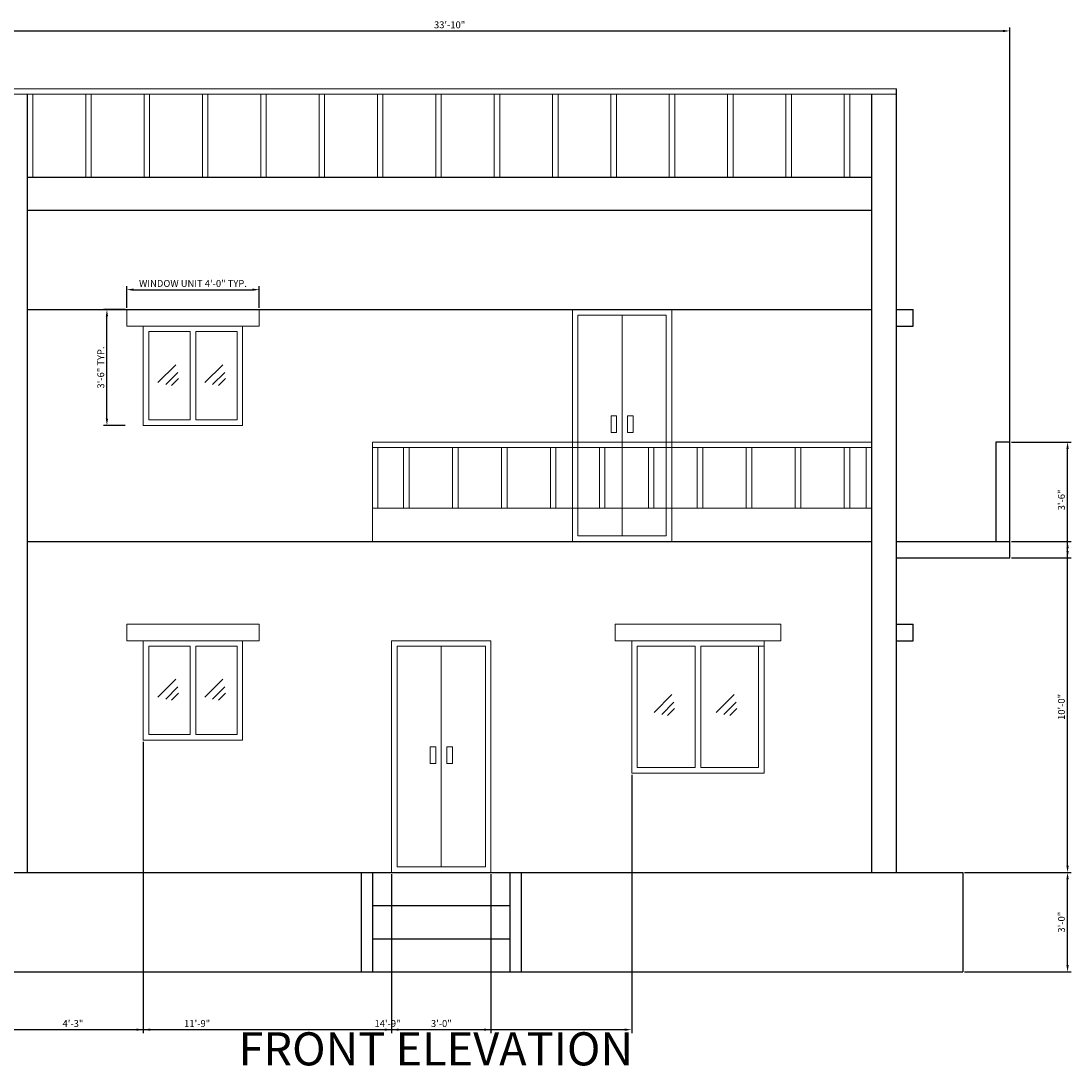
# Model space of a CAD drawing. Units: inches. Extents: x 2443635 to 2446153, y 1826255 to 1827341.
# Tile 16 of 16: x 2445772 to 2446153, y 1826829 to 1827207. Entities that reach past the tile are written whole.
import ezdxf

# ---------------------------------------------------------------- set-up
doc = ezdxf.new("R2010")
doc.units = ezdxf.units.IN
for name, color, linetype, lineweight in [('A-DIMS', 1, 'Continuous', 18), ('A-ELEV', 7, 'Continuous', 25), ('A-ELEV-DOOR', 2, 'Continuous', 18), ('A-ELEV-GLAZ', 4, 'Continuous', 18), ('A-ELEV-RAIL', 9, 'Continuous', 18), ('A-TEXT', 4, 'Continuous', 25)]:
    doc.layers.add(name, color=color, linetype=linetype, lineweight=lineweight)
doc.styles.get("Standard").update_dxf_attribs({"font": 'arial.ttf'})
doc.dimstyles.new('ISO-25', dxfattribs={"dimtxt": 2.5, "dimasz": 2.5, "dimexe": 1.25, "dimexo": 0.625, "dimtad": 1, "dimlunit": 4, "dimtxsty": 'Standard', "dimcen": 2.5, "dimadec": 0, "dimazin": 0, "dimtfac": 1, "dimtmove": 0, "dimatfit": 3, "dimfxl": 1, "dimarcsym": 0})

# ---------------------------------------------------------------- blocks, each defined once
blk = doc.blocks.new('WINDOW-36-ELEV')
at = {"transparency": 33554687}
for p, q in [((48, 42), (0, 42)), ((0, 36), (0, 42)), ((48, 36), (48, 42)), ((48, 36), (0, 36)), ((6, 0), (6, 36)), ((42, 36), (42, 0)), ((8, 2), (8, 34)), ((23, 34), (8, 34)), ((23, 2), (23, 34)), ((40, 34), (25, 34)), ((25, 2), (25, 34)), ((40, 34), (40, 2)), ((17.76, 22), (11.31, 15.54)), ((18.51, 19.22), (14.11, 14.82)), ((34.78, 22), (28.32, 15.54)), ((35.53, 19.22), (31.13, 14.82)), ((18.76, 16.98), (16.23, 14.45)), ((35.77, 16.98), (33.24, 14.45)), ((42, 0), (6, 0)), ((23, 2), (8, 2)), ((40, 2), (25, 2))]:
    blk.add_line(p, q, dxfattribs=at)
blk = doc.blocks.new('*D78')
at = {"layer": 'A-DIMS', "color": 0, "lineweight": -2, "transparency": 16777216}
for p, q in [((2445810.56, 1827103.33), (2445810.56, 1827111.15)), ((2445813.06, 1827109.9), (2445856.06, 1827109.9)), ((2445858.56, 1827103.33), (2445858.56, 1827111.15))]:
    blk.add_line(p, q, dxfattribs=at)
at = {"layer": 'A-DIMS', "color": 0, "transparency": 16777216}
for points in [[(2445813.06, 1827110.32), (2445813.06, 1827109.48), (2445810.56, 1827109.9)], [(2445856.06, 1827110.32), (2445856.06, 1827109.48), (2445858.56, 1827109.9)]]:
    blk.add_solid(points, dxfattribs=at)
at = {"layer": 'Defpoints', "color": 0, "transparency": 16777216}
for p in [(2445858.56, 1827109.9), (2445810.56, 1827102.7), (2445858.56, 1827102.7)]:
    blk.add_point(p, dxfattribs=at)
at = {"layer": 'A-DIMS', "color": 0, "transparency": 16777216, "insert": (2445834.56, 1827111.82), "char_height": 2.5, "attachment_point": 5}
blk.add_mtext('WINDOW UNIT 4\'-0" TYP.', dxfattribs=at)
blk = doc.blocks.new('*D79')
at = {"layer": 'A-DIMS', "color": 0, "lineweight": -2, "transparency": 16777216}
for p, q in [((2445809.93, 1827102.7), (2445802.11, 1827102.7)), ((2445803.36, 1827063.2), (2445803.36, 1827100.2)), ((2445809.93, 1827060.7), (2445802.11, 1827060.7))]:
    blk.add_line(p, q, dxfattribs=at)
at = {"layer": 'A-DIMS', "color": 0, "transparency": 16777216}
for points in [[(2445802.94, 1827100.2), (2445803.78, 1827100.2), (2445803.36, 1827102.7)], [(2445802.94, 1827063.2), (2445803.78, 1827063.2), (2445803.36, 1827060.7)]]:
    blk.add_solid(points, dxfattribs=at)
at = {"layer": 'Defpoints', "color": 0, "transparency": 16777216}
for p in [(2445803.36, 1827102.7), (2445810.56, 1827102.7), (2445810.56, 1827060.7)]:
    blk.add_point(p, dxfattribs=at)
at = {"layer": 'A-DIMS', "color": 0, "transparency": 16777216, "insert": (2445801.46, 1827081.7), "char_height": 2.5, "attachment_point": 5, "rotation": 90}
blk.add_mtext('3\'-6" TYP.', dxfattribs=at)
blk = doc.blocks.new('*D107')
at = {"layer": 'A-DIMS', "color": 0, "lineweight": -2, "transparency": 16777216}
for p, q in [((2445724.56, 1827013.33), (2445724.56, 1827204.9)), ((2446130.56, 1827013.33), (2446130.56, 1827204.9)), ((2445727.06, 1827203.65), (2446128.06, 1827203.65))]:
    blk.add_line(p, q, dxfattribs=at)
at = {"layer": 'A-DIMS', "color": 0, "transparency": 16777216}
for points in [[(2445727.06, 1827204.07), (2445727.06, 1827203.23), (2445724.56, 1827203.65)], [(2446128.06, 1827204.07), (2446128.06, 1827203.23), (2446130.56, 1827203.65)]]:
    blk.add_solid(points, dxfattribs=at)
at = {"layer": 'Defpoints', "color": 0, "transparency": 16777216}
for p in [(2446130.56, 1827203.65), (2445724.56, 1827012.7), (2446130.56, 1827012.7)]:
    blk.add_point(p, dxfattribs=at)
at = {"layer": 'A-DIMS', "color": 0, "transparency": 16777216, "insert": (2445927.56, 1827205.55), "char_height": 2.5, "attachment_point": 5}
blk.add_mtext('33\'-10"', dxfattribs=at)
blk = doc.blocks.new('*D109')
at = {"layer": 'A-DIMS', "color": 0, "lineweight": -2, "transparency": 16777216}
for p, q in [((2445765.56, 1826898.08), (2445765.56, 1826840.5)), ((2445906.56, 1826898.08), (2445906.56, 1826840.5)), ((2445768.06, 1826841.75), (2445904.06, 1826841.75))]:
    blk.add_line(p, q, dxfattribs=at)
at = {"layer": 'A-DIMS', "color": 0, "transparency": 16777216}
for points in [[(2445768.06, 1826842.17), (2445768.06, 1826841.33), (2445765.56, 1826841.75)], [(2445904.06, 1826842.17), (2445904.06, 1826841.33), (2445906.56, 1826841.75)]]:
    blk.add_solid(points, dxfattribs=at)
at = {"layer": 'Defpoints', "color": 0, "transparency": 16777216}
for p in [(2445765.56, 1826898.7), (2445906.56, 1826898.7), (2445906.56, 1826841.75)]:
    blk.add_point(p, dxfattribs=at)
at = {"layer": 'A-DIMS', "color": 0, "transparency": 16777216, "insert": (2445836.06, 1826843.65), "char_height": 2.5, "attachment_point": 5}
blk.add_mtext('11\'-9"', dxfattribs=at)
blk = doc.blocks.new('*D110')
at = {"layer": 'A-DIMS', "color": 0, "lineweight": -2, "transparency": 16777216}
for p, q in [((2445906.56, 1826898.08), (2445906.56, 1826840.5)), ((2445942.56, 1826898.08), (2445942.56, 1826840.5)), ((2445909.06, 1826841.75), (2445940.06, 1826841.75))]:
    blk.add_line(p, q, dxfattribs=at)
at = {"layer": 'A-DIMS', "color": 0, "transparency": 16777216}
for points in [[(2445909.06, 1826842.17), (2445909.06, 1826841.33), (2445906.56, 1826841.75)], [(2445940.06, 1826842.17), (2445940.06, 1826841.33), (2445942.56, 1826841.75)]]:
    blk.add_solid(points, dxfattribs=at)
at = {"layer": 'Defpoints', "color": 0, "transparency": 16777216}
for p in [(2445906.56, 1826898.7), (2445942.56, 1826898.7), (2445942.56, 1826841.75)]:
    blk.add_point(p, dxfattribs=at)
at = {"layer": 'A-DIMS', "color": 0, "transparency": 16777216, "insert": (2445924.56, 1826843.65), "char_height": 2.5, "attachment_point": 5}
blk.add_mtext('3\'-0"', dxfattribs=at)
blk = doc.blocks.new('*D111')
at = {"layer": 'A-DIMS', "color": 0, "lineweight": -2, "transparency": 16777216}
for p, q in [((2445816.56, 1826946.08), (2445816.56, 1826840.5)), ((2445765.56, 1826898.08), (2445765.56, 1826840.5)), ((2445768.06, 1826841.75), (2445814.06, 1826841.75))]:
    blk.add_line(p, q, dxfattribs=at)
at = {"layer": 'A-DIMS', "color": 0, "transparency": 16777216}
for points in [[(2445768.06, 1826842.17), (2445768.06, 1826841.33), (2445765.56, 1826841.75)], [(2445814.06, 1826842.17), (2445814.06, 1826841.33), (2445816.56, 1826841.75)]]:
    blk.add_solid(points, dxfattribs=at)
at = {"layer": 'Defpoints', "color": 0, "transparency": 16777216}
for p in [(2445816.56, 1826946.7), (2445765.56, 1826898.7), (2445816.56, 1826841.75)]:
    blk.add_point(p, dxfattribs=at)
at = {"layer": 'A-DIMS', "color": 0, "transparency": 16777216, "insert": (2445791.06, 1826843.65), "char_height": 2.5, "attachment_point": 5}
blk.add_mtext('4\'-3"', dxfattribs=at)
blk = doc.blocks.new('*D112')
at = {"layer": 'A-DIMS', "color": 0, "lineweight": -2, "transparency": 16777216}
for p, q in [((2445816.56, 1826946.08), (2445816.56, 1826840.5)), ((2445993.56, 1826934.08), (2445993.56, 1826840.5)), ((2445819.06, 1826841.75), (2445991.06, 1826841.75))]:
    blk.add_line(p, q, dxfattribs=at)
at = {"layer": 'A-DIMS', "color": 0, "transparency": 16777216}
for points in [[(2445819.06, 1826842.17), (2445819.06, 1826841.33), (2445816.56, 1826841.75)], [(2445991.06, 1826842.17), (2445991.06, 1826841.33), (2445993.56, 1826841.75)]]:
    blk.add_solid(points, dxfattribs=at)
at = {"layer": 'Defpoints', "color": 0, "transparency": 16777216}
for p in [(2445816.56, 1826946.7), (2445993.56, 1826934.7), (2445993.56, 1826841.75)]:
    blk.add_point(p, dxfattribs=at)
at = {"layer": 'A-DIMS', "color": 0, "transparency": 16777216, "insert": (2445905.06, 1826843.65), "char_height": 2.5, "attachment_point": 5}
blk.add_mtext('14\'-9"', dxfattribs=at)
blk = doc.blocks.new('*D113')
at = {"layer": 'A-DIMS', "color": 0, "lineweight": -2, "transparency": 16777216}
for p, q in [((2446114.18, 1826898.7), (2446152.76, 1826898.7)), ((2446151.51, 1826865.2), (2446151.51, 1826896.2)), ((2446114.18, 1826862.7), (2446152.76, 1826862.7))]:
    blk.add_line(p, q, dxfattribs=at)
at = {"layer": 'A-DIMS', "color": 0, "transparency": 16777216}
for points in [[(2446151.09, 1826896.2), (2446151.93, 1826896.2), (2446151.51, 1826898.7)], [(2446151.09, 1826865.2), (2446151.93, 1826865.2), (2446151.51, 1826862.7)]]:
    blk.add_solid(points, dxfattribs=at)
at = {"layer": 'Defpoints', "color": 0, "transparency": 16777216}
for p in [(2446113.56, 1826898.7), (2446151.51, 1826898.7), (2446113.56, 1826862.7)]:
    blk.add_point(p, dxfattribs=at)
at = {"layer": 'A-DIMS', "color": 0, "transparency": 16777216, "insert": (2446149.61, 1826880.7), "char_height": 2.5, "attachment_point": 5, "rotation": 90}
blk.add_mtext('3\'-0"', dxfattribs=at)
blk = doc.blocks.new('*D114')
at = {"layer": 'A-DIMS', "color": 0, "lineweight": -2, "transparency": 16777216}
for p, q in [((2446131.18, 1827054.7), (2446152.76, 1827054.7)), ((2446151.51, 1827015.2), (2446151.51, 1827052.2)), ((2446131.18, 1827012.7), (2446152.76, 1827012.7))]:
    blk.add_line(p, q, dxfattribs=at)
at = {"layer": 'A-DIMS', "color": 0, "transparency": 16777216}
for points in [[(2446151.09, 1827052.2), (2446151.93, 1827052.2), (2446151.51, 1827054.7)], [(2446151.09, 1827015.2), (2446151.93, 1827015.2), (2446151.51, 1827012.7)]]:
    blk.add_solid(points, dxfattribs=at)
at = {"layer": 'Defpoints', "color": 0, "transparency": 16777216}
for p in [(2446130.56, 1827054.7), (2446151.51, 1827054.7), (2446130.56, 1827012.7)]:
    blk.add_point(p, dxfattribs=at)
at = {"layer": 'A-DIMS', "color": 0, "transparency": 16777216, "insert": (2446149.61, 1827033.7), "char_height": 2.5, "attachment_point": 5, "rotation": 90}
blk.add_mtext('3\'-6"', dxfattribs=at)
blk = doc.blocks.new('*D115')
at = {"layer": 'A-DIMS', "color": 0, "lineweight": -2, "transparency": 16777216}
for p, q in [((2446131.18, 1827018.7), (2446152.76, 1827018.7)), ((2446151.51, 1826901.2), (2446151.51, 1827016.2)), ((2446114.18, 1826898.7), (2446152.76, 1826898.7))]:
    blk.add_line(p, q, dxfattribs=at)
at = {"layer": 'A-DIMS', "color": 0, "transparency": 16777216}
for points in [[(2446151.09, 1827016.2), (2446151.93, 1827016.2), (2446151.51, 1827018.7)], [(2446151.09, 1826901.2), (2446151.93, 1826901.2), (2446151.51, 1826898.7)]]:
    blk.add_solid(points, dxfattribs=at)
at = {"layer": 'Defpoints', "color": 0, "transparency": 16777216}
for p in [(2446130.56, 1827018.7), (2446151.51, 1827018.7), (2446113.56, 1826898.7)]:
    blk.add_point(p, dxfattribs=at)
at = {"layer": 'A-DIMS', "color": 0, "transparency": 16777216, "insert": (2446149.61, 1826958.7), "char_height": 2.5, "attachment_point": 5, "rotation": 90}
blk.add_mtext('10\'-0"', dxfattribs=at)

msp = doc.modelspace()

# ---------------------------------------------------------------- linework, layer by layer
at = {"layer": 'A-ELEV'}
for p, q in [((2446089.56, 1826898.701), (2446089.56, 1827182.701)), ((2445774.56, 1826898.701), (2445774.56, 1827180.701)), ((2446080.56, 1826898.701), (2446080.56, 1827180.701)), ((2445858.56, 1827102.701), (2446080.56, 1827102.701)), ((2445741.56, 1826898.701), (2446113.56, 1826898.701)), ((2445895.56, 1826898.701), (2445895.56, 1826862.701)), ((2445899.56, 1826898.701), (2445899.56, 1826862.701)), ((2445949.56, 1826862.701), (2445949.56, 1826898.701)), ((2445953.56, 1826862.701), (2445953.56, 1826898.701)), ((2445899.56, 1826886.701), (2445949.56, 1826886.701)), ((2445899.56, 1826874.701), (2445949.56, 1826874.701)), ((2445741.56, 1826862.701), (2446113.56, 1826862.701))]:
    msp.add_line(p, q, dxfattribs=at)
at = {"layer": 'A-ELEV', "transparency": 33554687}
for p, q in [((2445774.56, 1827150.701), (2446080.56, 1827150.701)), ((2445774.56, 1827138.701), (2446080.56, 1827138.701)), ((2445774.56, 1827102.701), (2445810.56, 1827102.701)), ((2445774.56, 1827102.701), (2446080.56, 1827102.701)), ((2446089.56, 1827102.701), (2446095.56, 1827102.701)), ((2446095.56, 1827096.701), (2446095.56, 1827102.701)), ((2446089.56, 1827096.701), (2446095.56, 1827096.701)), ((2446130.56, 1827054.701), (2446125.56, 1827054.701)), ((2446125.56, 1827054.701), (2446125.56, 1827018.701)), ((2446130.56, 1827012.701), (2446130.56, 1827054.701)), ((2445774.56, 1827018.701), (2446080.56, 1827018.701)), ((2446089.56, 1827018.701), (2446130.56, 1827018.701)), ((2446089.56, 1827012.701), (2446130.56, 1827012.701)), ((2446089.56, 1826988.701), (2446095.56, 1826988.701)), ((2446095.56, 1826982.701), (2446095.56, 1826988.701)), ((2446089.56, 1826982.701), (2446095.56, 1826982.701)), ((2446113.56, 1826898.701), (2446113.56, 1826862.701))]:
    msp.add_line(p, q, dxfattribs=at)
at = {"layer": 'A-ELEV-DOOR'}
for p, q in [((2445972.06, 1827054.701), (2445972.06, 1827102.701)), ((2446008.06, 1827102.701), (2445972.06, 1827102.701)), ((2446008.06, 1827054.701), (2446008.06, 1827102.701)), ((2445974.06, 1827100.701), (2446006.06, 1827100.701)), ((2445974.06, 1827054.701), (2445974.06, 1827100.701)), ((2445990.06, 1827100.701), (2445990.06, 1827054.701)), ((2446006.06, 1827054.701), (2446006.06, 1827100.701)), ((2445986.06, 1827064.201), (2445986.06, 1827058.201)), ((2445988.06, 1827064.201), (2445986.06, 1827064.201)), ((2445988.06, 1827064.201), (2445988.06, 1827058.201)), ((2445992.06, 1827064.201), (2445992.06, 1827058.201)), ((2445992.06, 1827064.201), (2445994.06, 1827064.201)), ((2445994.06, 1827064.201), (2445994.06, 1827058.201)), ((2445988.06, 1827058.201), (2445986.06, 1827058.201)), ((2445992.06, 1827058.201), (2445994.06, 1827058.201)), ((2446008.06, 1827054.701), (2445972.06, 1827054.701)), ((2445906.56, 1826898.701), (2445906.56, 1826982.701)), ((2445942.56, 1826982.701), (2445906.56, 1826982.701)), ((2445908.56, 1826900.701), (2445908.56, 1826980.701)), ((2445908.56, 1826980.701), (2445940.56, 1826980.701)), ((2445924.56, 1826980.701), (2445924.56, 1826900.701)), ((2445940.56, 1826900.701), (2445940.56, 1826980.701)), ((2445942.56, 1826898.701), (2445942.56, 1826982.701)), ((2445920.56, 1826944.201), (2445920.56, 1826938.201)), ((2445922.56, 1826944.201), (2445920.56, 1826944.201)), ((2445922.56, 1826944.201), (2445922.56, 1826938.201)), ((2445926.56, 1826944.201), (2445926.56, 1826938.201)), ((2445926.56, 1826944.201), (2445928.56, 1826944.201)), ((2445928.56, 1826944.201), (2445928.56, 1826938.201)), ((2445922.56, 1826938.201), (2445920.56, 1826938.201)), ((2445926.56, 1826938.201), (2445928.56, 1826938.201)), ((2445908.56, 1826900.701), (2445940.56, 1826900.701))]:
    msp.add_line(p, q, dxfattribs=at)
at = {"layer": 'A-ELEV-DOOR', "transparency": 33554559}
for p, q in [((2445972.06, 1827018.701), (2445972.06, 1827054.701)), ((2445974.06, 1827020.701), (2445974.06, 1827054.701)), ((2445990.06, 1827054.701), (2445990.06, 1827020.701)), ((2446006.06, 1827020.701), (2446006.06, 1827054.701)), ((2446008.06, 1827018.701), (2446008.06, 1827054.701)), ((2445972.06, 1827018.701), (2446008.06, 1827018.701)), ((2445974.06, 1827020.701), (2446006.06, 1827020.701))]:
    msp.add_line(p, q, dxfattribs=at)
at = {"layer": 'A-ELEV-GLAZ'}
for p, q in [((2445987.56, 1826988.701), (2446047.56, 1826988.701)), ((2445987.56, 1826988.701), (2445987.56, 1826982.701)), ((2446047.56, 1826982.701), (2446047.56, 1826988.701)), ((2445987.56, 1826982.701), (2446047.56, 1826982.701)), ((2445993.56, 1826934.701), (2445993.56, 1826982.701)), ((2445995.56, 1826936.701), (2445995.56, 1826980.701)), ((2445995.56, 1826980.701), (2446016.56, 1826980.701)), ((2446016.56, 1826980.701), (2446016.56, 1826936.701)), ((2446018.56, 1826980.701), (2446018.56, 1826936.701)), ((2446018.56, 1826980.701), (2446041.56, 1826980.701)), ((2446039.56, 1826936.701), (2446039.56, 1826980.701)), ((2446041.56, 1826934.701), (2446041.56, 1826982.701)), ((2446008.102, 1826963.153), (2446001.645, 1826956.696)), ((2446030.649, 1826963.153), (2446024.192, 1826956.696)), ((2446008.847, 1826960.372), (2446004.451, 1826955.977)), ((2446009.095, 1826958.138), (2446006.562, 1826955.605)), ((2446031.394, 1826960.372), (2446026.999, 1826955.977)), ((2446031.642, 1826958.138), (2446029.109, 1826955.605)), ((2445993.56, 1826934.701), (2446041.56, 1826934.701)), ((2445995.56, 1826936.701), (2446016.56, 1826936.701)), ((2446018.56, 1826936.701), (2446039.56, 1826936.701))]:
    msp.add_line(p, q, dxfattribs=at)
at = {"layer": 'A-ELEV-RAIL', "transparency": 33554687}
for p, q in [((2445765.56, 1827182.701), (2446089.56, 1827182.701)), ((2445765.56, 1827180.701), (2446089.56, 1827180.701)), ((2445774.56, 1827150.701), (2445774.56, 1827180.701)), ((2445776.56, 1827150.701), (2445776.56, 1827180.701)), ((2445795.703, 1827150.701), (2445795.703, 1827180.701)), ((2445797.703, 1827150.701), (2445797.703, 1827180.701)), ((2445816.845, 1827150.701), (2445816.845, 1827180.701)), ((2445818.845, 1827150.701), (2445818.845, 1827180.701)), ((2445837.988, 1827150.701), (2445837.988, 1827180.701)), ((2445839.988, 1827150.701), (2445839.988, 1827180.701)), ((2445859.131, 1827150.701), (2445859.131, 1827180.701)), ((2445861.131, 1827150.701), (2445861.131, 1827180.701)), ((2445880.274, 1827150.701), (2445880.274, 1827180.701)), ((2445882.274, 1827150.701), (2445882.274, 1827180.701)), ((2445901.417, 1827150.701), (2445901.417, 1827180.701)), ((2445903.417, 1827150.701), (2445903.417, 1827180.701)), ((2445922.56, 1827150.701), (2445922.56, 1827180.701)), ((2445924.56, 1827150.701), (2445924.56, 1827180.701)), ((2445943.703, 1827150.701), (2445943.703, 1827180.701)), ((2445945.703, 1827150.701), (2445945.703, 1827180.701)), ((2445964.845, 1827150.701), (2445964.845, 1827180.701)), ((2445966.845, 1827150.701), (2445966.845, 1827180.701)), ((2445985.988, 1827150.701), (2445985.988, 1827180.701)), ((2445987.988, 1827150.701), (2445987.988, 1827180.701)), ((2446007.131, 1827150.701), (2446007.131, 1827180.701)), ((2446009.131, 1827150.701), (2446009.131, 1827180.701)), ((2446028.274, 1827150.701), (2446028.274, 1827180.701)), ((2446030.274, 1827150.701), (2446030.274, 1827180.701)), ((2446049.417, 1827150.701), (2446049.417, 1827180.701)), ((2446051.417, 1827150.701), (2446051.417, 1827180.701)), ((2446070.56, 1827150.701), (2446070.56, 1827180.701)), ((2446072.56, 1827150.701), (2446072.56, 1827180.701))]:
    msp.add_line(p, q, dxfattribs=at)
at = {"layer": 'A-ELEV-RAIL'}
for p, q in [((2445899.56, 1827018.701), (2445899.56, 1827054.701)), ((2445899.56, 1827054.701), (2446080.56, 1827054.701)), ((2445899.56, 1827052.701), (2446080.56, 1827052.701)), ((2445901.56, 1827030.701), (2445901.56, 1827052.701)), ((2445910.89, 1827030.701), (2445910.89, 1827052.701)), ((2445912.89, 1827030.701), (2445912.89, 1827052.701)), ((2445928.631, 1827030.701), (2445928.631, 1827052.701)), ((2445930.631, 1827030.701), (2445930.631, 1827052.701)), ((2445946.372, 1827030.701), (2445946.372, 1827052.701)), ((2445948.372, 1827030.701), (2445948.372, 1827052.701)), ((2445964.113, 1827030.701), (2445964.113, 1827052.701)), ((2445966.113, 1827030.701), (2445966.113, 1827052.701)), ((2445981.854, 1827030.701), (2445981.854, 1827052.701)), ((2445983.854, 1827030.701), (2445983.854, 1827052.701)), ((2445999.595, 1827030.701), (2445999.595, 1827052.701)), ((2446001.595, 1827030.701), (2446001.595, 1827052.701)), ((2446017.336, 1827030.701), (2446017.336, 1827052.701)), ((2446019.336, 1827030.701), (2446019.336, 1827052.701)), ((2446035.077, 1827030.701), (2446035.077, 1827052.701)), ((2446037.077, 1827030.701), (2446037.077, 1827052.701)), ((2446052.819, 1827030.701), (2446052.819, 1827052.701)), ((2446054.819, 1827030.701), (2446054.819, 1827052.701)), ((2446070.56, 1827030.701), (2446070.56, 1827052.701)), ((2446072.56, 1827030.701), (2446072.56, 1827052.701)), ((2446078.56, 1827030.701), (2446078.56, 1827052.701)), ((2446080.56, 1827018.701), (2446080.56, 1827054.701)), ((2445899.56, 1827030.701), (2446080.56, 1827030.701))]:
    msp.add_line(p, q, dxfattribs=at)

# ---------------------------------------------------------------- block references
at = {"layer": 'A-ELEV-GLAZ', "transparency": 33554687}
for p in [(2445810.56, 1827060.701), (2445810.56, 1826946.701)]:
    msp.add_blockref('WINDOW-36-ELEV', p, dxfattribs=at)

# ---------------------------------------------------------------- texts
at = {"layer": 'A-TEXT', "transparency": 33554687, "insert": (2445851.045, 1826840.797), "char_height": 12, "attachment_point": 1}
msp.add_mtext_dynamic_manual_height_columns('FRONT ELEVATION', width=201.69861, gutter_width=12.5, heights=[0], dxfattribs=at)

# ---------------------------------------------------------------- dimensions: what is measured, and where the dimension line sits
at = {"layer": 'A-DIMS', "transparency": 33554687}
for base, p1, p2, picture, middle in [((2446130.56, 1827203.651), (2445724.56, 1827012.701), (2446130.56, 1827012.701), '*D107', (2445927.56, 1827205.553)), ((2445816.56, 1826841.751), (2445765.56, 1826898.701), (2445816.56, 1826946.701), '*D111', (2445791.06, 1826843.653)), ((2445993.56, 1826841.751), (2445816.56, 1826946.701), (2445993.56, 1826934.701), '*D112', (2445905.06, 1826843.653)), ((2445906.56, 1826841.751), (2445765.56, 1826898.701), (2445906.56, 1826898.701), '*D109', (2445836.06, 1826843.653)), ((2445942.56, 1826841.751), (2445906.56, 1826898.701), (2445942.56, 1826898.701), '*D110', (2445924.56, 1826843.653))]:
    dim = msp.add_linear_dim(base=base, p1=p1, p2=p2, dimstyle='ISO-25', override={"dimdec": 1, "dimlfac": 1, "dimrnd": 0, "dimzin": 1, "dimdsep": 46, "dimlunit": 4, "dimfrac": 2}, dxfattribs=at)
    dim.commit()
    dim.dimension.update_dxf_attribs({"geometry": picture, "text_midpoint": middle})
dim = msp.add_linear_dim(base=(2445858.56, 1827109.901), p1=(2445810.56, 1827102.701), p2=(2445858.56, 1827102.701), text='WINDOW UNIT <> TYP.', dimstyle='ISO-25', override={"dimdec": 1, "dimlfac": 1, "dimrnd": 0, "dimzin": 1, "dimdsep": 46, "dimlunit": 4, "dimfrac": 2}, dxfattribs=at)
dim.commit()
dim.dimension.update_dxf_attribs({"geometry": '*D78', "text_midpoint": (2445834.56, 1827111.82)})
dim = msp.add_linear_dim(base=(2445803.36, 1827102.701), p1=(2445810.56, 1827060.701), p2=(2445810.56, 1827102.701), angle=90, text='<> TYP.', dimstyle='ISO-25', override={"dimdec": 1, "dimlfac": 1, "dimrnd": 0, "dimzin": 1, "dimdsep": 46, "dimlunit": 4, "dimfrac": 2}, dxfattribs=at)
dim.commit()
dim.dimension.update_dxf_attribs({"geometry": '*D79', "text_midpoint": (2445801.457, 1827081.701)})
for base, p1, p2, picture, middle in [((2446151.51, 1827054.701), (2446130.56, 1827012.701), (2446130.56, 1827054.701), '*D114', (2446149.607, 1827033.701)), ((2446151.51, 1827018.701), (2446113.56, 1826898.701), (2446130.56, 1827018.701), '*D115', (2446149.608, 1826958.701)), ((2446151.51, 1826898.701), (2446113.56, 1826862.701), (2446113.56, 1826898.701), '*D113', (2446149.607, 1826880.701))]:
    dim = msp.add_linear_dim(base=base, p1=p1, p2=p2, angle=90, dimstyle='ISO-25', override={"dimdec": 1, "dimlfac": 1, "dimrnd": 0, "dimzin": 1, "dimdsep": 46, "dimlunit": 4, "dimfrac": 2}, dxfattribs=at)
    dim.commit()
    dim.dimension.update_dxf_attribs({"geometry": picture, "text_midpoint": middle})

doc.saveas('drawing.dxf')
